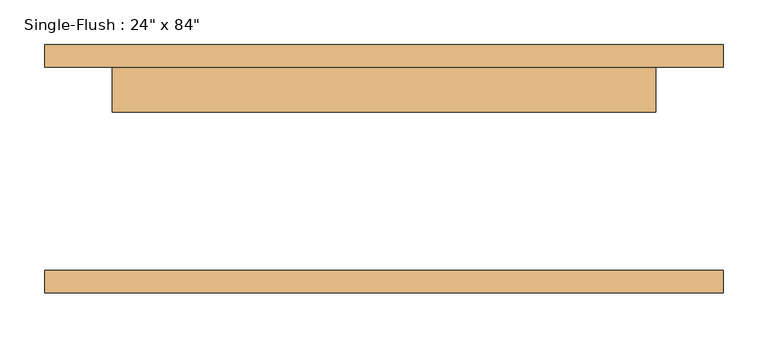
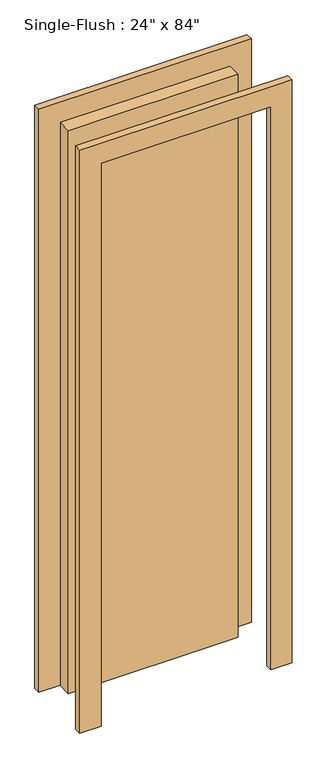
"""IFC4 building model written with IfcOpenShell, lengths in millimetres: door geometry."""

from ifc_helpers import new_model, si_unit, frame, origin, origin_with_axes, place, context, project, spatial, polyline, outline, extrude, source, transform, mapped, element, save


def door_0d3b4037(model_context):
    return source(origin(), model_context, "Body", "SweptSolid", [
        extrude(outline(polyline([(2209.8, -381.0), (0.0, -381.0), (0.0, -304.8), (2133.6, -304.8), (2133.6, 304.8), (0.0, 304.8), (0.0, 381.0), (2209.8, 381.0), (2209.8, -381.0)])), frame((0.0, 114.3, 0.0), z_axis=(0.0, 1.0, 0.0), x_axis=(0.0, 0.0, 1.0)), (0.0, 0.0, 1.0), 25.4),
        extrude(outline(polyline([(2209.8, 381.0), (2209.8, -381.0), (0.0, -381.0), (0.0, -304.8), (2133.6, -304.8), (2133.6, 304.8), (0.0, 304.8), (0.0, 381.0), (2209.8, 381.0)])), frame((0.0, -139.7, 0.0), z_axis=(0.0, 1.0, 0.0), x_axis=(0.0, 0.0, 1.0)), (0.0, 0.0, 1.0), 25.4),
        extrude(outline(polyline([(304.8, 63.5), (-304.8, 63.5), (-304.8, 114.3), (304.8, 114.3), (304.8, 63.5)])), origin_with_axes(), (0.0, 0.0, 1.0), 2133.6),
    ])


if __name__ == "__main__":
    model = new_model("IFC4")
    model_context = context("Model", 3, world=origin())
    ifc_project = project(units=[si_unit("LENGTHUNIT", "METRE", prefix="MILLI")], contexts=[model_context])
    site = spatial("IfcSite", under=ifc_project)
    building = spatial("IfcBuilding", under=site)
    placement = place(None, origin())
    door_shape = door_0d3b4037(model_context)
    element("IfcDoor", 1, ObjectType="Single-Flush : 24\" x 84\"", at=placement, inside=building, context=model_context, shape_type="MappedRepresentation", body=[
        mapped(door_shape, transform((0.0, 0.0, 0.0), x_axis=(1.0, 0.0, 0.0), y_axis=(0.0, 1.0, 0.0), z_axis=(0.0, 0.0, 1.0))),
    ])
    save(model, "model.ifc")

# Revit data of these elements
# Type "Single-Flush : 24\" x 84\""
#   Type Mark = "1"
#   Construction Type Id = "MDOOR"
#   Assembly Code = "C1020"
#   Analytic Construction = "Metal"
#   Thickness = 0' - 2"
#   Heat Transfer Coefficient (U) = 0.651978 BTU/(h·ft²·°F)
#   Height = 7' - 0"
#   Trim Projection Ext = 0' - 1"
#   Trim Projection Int = 0' - 1"
#   Trim Width = 0' - 3"
#   Width = 2' - 0"
#   Define Thermal Properties by = 1
#   Define Thermal Properties by = 1
#   Door Material = Door - Panel
#   Frame Material = Door - Frame
#   Visual Light Transmittance = 0
#   Solar Heat Gain Coefficient = 0
#   Function = (empty or 0)
#   Wall Closure = (empty or 0)
# Element 1 (IfcDoor, "Single-Flush : 24\" x 84\"")
#   Materials on its faces: "Door - Frame", "Door - Panel"
# Materials
#   "Door - Panel": class "Wood", colour RGB 210 159 95, transparency 0, Cost = 0
#   "Door - Frame": colour RGB 118 70 51, transparency 0, Cost = 0
